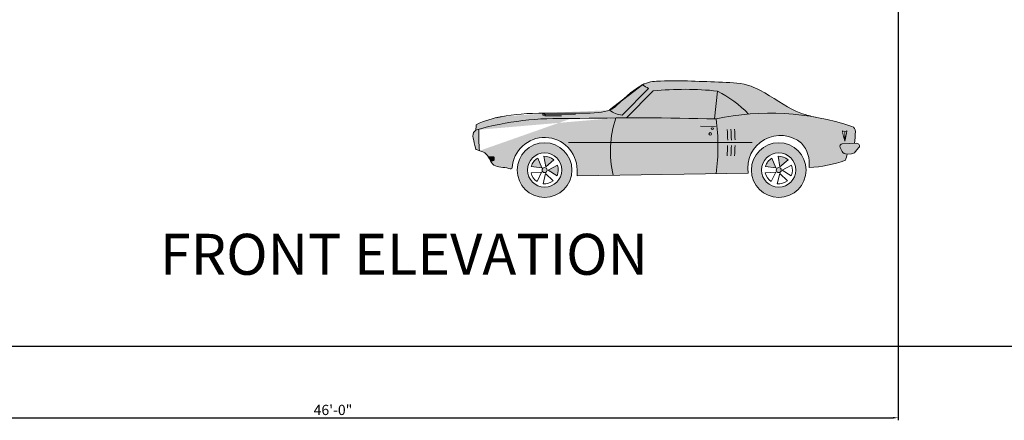
# Model space of a CAD drawing. Units: inches. Extents: x 1662 to 23131, y 1265 to 19127.
# Tile 22 of 26: x 22111 to 22592, y 17831 to 18027. Entities that reach past the tile are written whole.
import ezdxf

# ---------------------------------------------------------------- set-up
doc = ezdxf.new("R2010")
doc.units = ezdxf.units.IN
for name, color, linetype, lineweight in [('A-ANNO-DIMS', 4, 'Continuous', 18), ('A-ANNO-TITL', 7, 'Continuous', 35), ('A-ANNO-TTLB', 7, 'Continuous', 25), ('A-ELEV', 7, 'Continuous', 25), ('A-ELEV-SURF-PATT', 252, 'Continuous', 13), ('A-SITE-VEHC', 8, 'Continuous', 18)]:
    doc.layers.add(name, color=color, linetype=linetype, lineweight=lineweight)
doc.styles.get("Standard").update_dxf_attribs({"font": 'arial.ttf'})
doc.dimstyles.new('ISO-25', dxfattribs={"dimtxt": 5, "dimasz": 2.5, "dimexe": 1.25, "dimexo": 0.625, "dimtad": 1, "dimlunit": 3, "dimtxsty": 'Standard', "dimcen": 2.5, "dimadec": 0, "dimazin": 0, "dimtfac": 1, "dimtmove": 0, "dimatfit": 3, "dimfxl": 1, "dimarcsym": 0})

# ---------------------------------------------------------------- blocks, each defined once
blk = doc.blocks.new('*U125')
for p, q in [((1852.424305694587, 1021.94023515126), (2179.330987173972, 1350.645748622479)), ((1905.028754216457, 986.0402655627327), (2237.281665968954, 1320.121427396675)), ((3032.444313744444, 1318.435483164577), (2995.184084363387, 973.324104566919)), ((1273.239579640142, 1043.030435623248), (871.5032389472328, 1041.001834039635)), ((1098.89508774338, 1012.134004053351), (892.8883415085321, 1010.293803537071)), ((896.6541237575286, 1027.557353910195), (1273.36508552453, 1031.747823418233)), ((2821.704323889107, 882.1853508743229), (3009.40210199737, 879.9097921223942)), ((1184.937477293614, 681.4987119404606), (3461.750511828128, 679.9102527502469)), ((4554.181794982009, 618.5936445548908), (4578.428756696647, 571.2293072468502)), ((4581.292953023774, 664.6633678662108), (4762.788167963406, 670.807787640687)), ((4741.599689284432, 563.0499352002037), (4788.17251968349, 618.8856343936881)), ((189.2120355450149, 502.3517070685087), (247.4549749373119, 502.9995917502729)), ((4638.623553838175, 536.8785697564502), (4696.80346690226, 540.4040575811651)), ((247.9843470866509, 455.4105826600687), (216.7883795485336, 455.0635639533959)), ((263.4603752382749, 487.346356794033), (263.6375820428919, 471.4159829610306)), ((1292.174930811352, 343.511370615137), (1293.022509683079, 267.316507168658))]:
    blk.add_line(p, q)
for points in [[(896.8016502475936, 1014.295153612313), (896.7053017041424, 1022.956606081312, 0.2695324023286518), (892.630915434324, 1029.789683311358), (873.3170212489753, 1040.50624839506, 0.5753831854401361), (867.4395555695834, 1037.001668443855), (867.5359041130301, 1028.340215974855, 0.2695324023286636), (871.6102903828508, 1021.507138744809), (890.9241845682014, 1010.790573661109, 0.5753831854401859)], [(879.7836598367863, 509.3545565197219), (903.1759281139406, 380.3214176471538), (1003.225770169055, 465.0962856635947, 0.1999060696292243)], [(3784.383643640271, 509.3545565197196), (3807.775911917426, 380.3214176471517), (3907.82575397254, 465.0962856635924, 0.1999060696292243)], [(723.7168469426299, 383.4919578957729), (853.6632629200222, 365.8658943225199), (803.9546737544847, 487.2158234763112, 0.1999060696292243)], [(1047.713401858163, 399.8198790703183), (932.2242027500088, 337.699077145239), (1043.766994874665, 268.7428978173945, 0.1999060696292243)], [(3628.316830746115, 383.4919578957707), (3758.263246723507, 365.8658943225165), (3708.554657557972, 487.2158234763079, 0.1999060696292243)], [(3952.313385661648, 399.819879070315), (3836.824186553493, 337.6990771452344), (3948.366978678152, 268.7428978173922, 0.1999060696292243)], [(795.1919940795486, 196.1699165843778), (852.1110275926588, 314.3095490808095), (721.3395879004361, 304.5330618138037, 0.1999060696292243)], [(995.43287725522, 206.2611268358749), (900.664358595724, 296.9014987103449), (869.5517532737088, 169.5093681349639, 0.1999060696292243)], [(3699.791977883036, 196.1699165843755), (3756.711011396144, 314.3095490808073), (3625.939571703921, 304.5330618138014, 0.1999060696292243)], [(3900.032861058707, 206.2611268358726), (3805.264342399209, 296.9014987103415), (3774.151737077194, 169.5093681349606, 0.1999060696292243)]]:
    blk.add_lwpolyline(points, format="xyb", close=True)
for points in [[(4612.178408054545, 697.5855081472733), (4610.911620659674, 811.4659926516836), (4584.21673788074, 823.7136574833391)], [(4612.178408054545, 697.5855081472733), (4610.911620659674, 811.4659926516836), (4637.327449602523, 824.3044521259374)], [(1293.022509683079, 267.316507168658), (3413.278107073423, 300.3593556298297)]]:
    blk.add_lwpolyline(points)
for centre, radius in [((2943.507610451247, 787.54394792536), 15.73283948719639), ((888.3677559944676, 339.0194873812145), 339.0404618073459), ((3792.967739797953, 339.0194873812123), 339.0404618073459), ((888.3677559944676, 339.0194873812145), 212.1199727322649), ((3792.967739797953, 339.0194873812123), 212.1199727322649), ((888.3677559944631, 339.0194873812145), 31.6605939107037), ((3792.967739797948, 339.0194873812123), 31.6605939107037)]:
    blk.add_circle(centre, radius)
for centre, radius, start, end in [((2910.885371335993, 2669.23574072891), 1507.929501774574, 237.6102726860142, 240.9784649091492), ((2627.712114858283, -2413.041321416871), 3753.523683760239, 83.8163327171543, 95.97053738930742), ((2425.838500466955, 99.2748149861123), 1361.735417596019, 43.27478678783127, 63.56652369103386), ((1071.358229971631, -2828.229400839409), 3807.785853883705, 87.83927513879316, 105.8096485545998), ((521.544716666302, -80.01394318122811), 1093.607895506514, 98.53035379505096, 116.1119759439421), ((2034.516407361282, -34648.81188708144), 35635.08741385555, 88.42296055026361, 91.31789804800042), ((1861.480574200575, 1282.39025120185), 260.6074190425228, 230.4240102276009, 268.008535378073), ((3005.128481494482, 571.7965598232081), 1299.348755530903, 161.4307082840575, 193.2363327424058), ((3687.381330221874, -2156.074042366811), 3200.23423309803, 71.52833252843139, 102.1241928632375), ((651.7203661001014, 633.5641918017639), 2387.729331448684, 351.8278966526415, 8.167377222832604), ((4681.26729379385, 819.2266390839337), 63.32118782140739, 357.9320259294628, 71.5283325284308), ((2010.729354338346, 764.8379620713475), 1937.952811191957, 177.5773367925648, 185.5205157003238), ((888.3677559944676, 339.0194873812145), 403.8321575216381, 0.6373223477697438, 176.3412329397426), ((1159.222590401551, 681.5166523895871), 2000.491234107682, 0.8520117729178469, 4.65562176499107), ((1204.825955982183, 682.0239365738142), 2000.491234107682, 0.8520117729178469, 4.65562176499107), ((1250.429321562816, 682.5312207580412), 2000.491234107682, 0.8520117729178469, 4.65562176499107), ((3812.44326471366, 364.6726230309737), 404.3130216030247, 49.22630090364881, 189.1528042882995), ((5492.971123156516, 959.0142065914283), 918.7713379001904, 188.4683166415172, 196.5314518469167), ((3725.788185614365, 939.3563602145823), 918.7713379001904, 344.7431928486226, 352.806328054022), ((2960.464007730524, 881.3625008577552), 1785.245929105045, 353.1942286465509, 357.9320259294632), ((1159.222590401551, 681.5166523895871), 2000.491234107682, 355.2644314046092, 358.8632764442745), ((1204.825955982183, 682.0239365738142), 2000.491234107682, 355.2644314046092, 358.8632764442745), ((1250.429321562816, 682.5312207580412), 2000.491234107682, 355.2644314046092, 358.8632764442745), ((3794.827133462601, 420.2460268887999), 377.0136474469525, 352.7285496129741, 41.66131232724548), ((4582.364191149664, 633.0209018489084), 31.6605939107037, 91.93897627460323, 207.1090160995226), ((4763.859406089295, 639.1653216233844), 31.6605939107037, 320.168349060925, 91.93897627460312), ((247.6310576096746, 487.1702741216726), 15.83029695535184, 0.6373223477697438, 90.63732234776975), ((4634.793549031956, 600.0838218348852), 63.32118782140739, 207.1090160995214, 273.4676724156525), ((2901.892172686372, 940.4796147147171), 1785.245929105045, 344.3985036081313, 346.9384932927042), ((4692.973462096046, 603.6093096596), 63.32118782140739, 273.4676724156508, 320.168349060924), ((247.8082644142905, 471.239900288669), 15.83029695535184, 270.6373223477697, 0.6373223477697438), ((4126.811003434335, 1798.913596362007), 1427.004461663924, 271.6864966331125, 290.2773961774014)]:
    blk.add_arc(centre, radius, start, end)
blk.add_ellipse((2968.963243622841, 853.2791378181013), major_axis=(-16.00108995067517, -0.1779934388400297), ratio=0.6100431599522633)
for points, knots in [([(289.2906990761314, 988.6470416166414), (458.7737514417009, 1020.886061005622), (785.1067050195581, 1067.029451377599), (1645.088223183275, 1018.886905819271), (1784.344214682222, 1140.817014935552), (2091.760888566001, 1431.934919697545), (2519.289461757875, 1455.378874077572), (2948.002349952958, 1431.299395835894), (3379.283347368358, 1419.06290683643), (3689.197264561811, 1266.646942515618), (3901.855848393217, 1112.555284301348), (4093.662622991955, 1033.187703863597), (4189.021814386458, 1009.060173110094), (4249.111677936588, 994.4748246004747)], [18.62982323788346, 18.62982323788346, 18.62982323788346, 18.62982323788346, 19.52740456630144, 20.70057132475832, 21.10798274325262, 21.60856814090276, 21.92335951908455, 23.15135895041792, 23.71617100351322, 23.90874285473794, 24.77794011438314, 24.94307190945345, 25.1877551447545, 25.1877551447545, 25.1877551447545, 25.1877551447545]), ([(485.3586889456344, 364.7896896507493), (482.3269151854019, 360.8630236160399), (469.8642701632046, 350.8862285351804), (389.9323687006885, 380.8945308696264), (233.5219717046482, 354.0424667192036), (184.3560220232451, 564.4315200693248), (76.52041888637723, 575.4467616401544), (33.56437062048743, 599.7488008360459), (16.25711196136743, 683.7323555854283), (-24.37278573086193, 799.8748641589713), (39.13505772293892, 828.9834370117921), (38.00494619388845, 865.2204137053852), (37.84050808420068, 883.8077013151833), (37.78154551397344, 890.4725447213818), (38.61308557628376, 896.5033010551641), (40.21850136081582, 901.9755188649158)], [16.81585287302304, 16.81585287302304, 16.81585287302304, 16.81585287302304, 16.838212158335, 16.88539481137264, 17.18439046154897, 17.47984636192869, 17.65442317330994, 17.67069277424245, 17.69692296666891, 18.01635806820882, 18.05273947455308, 18.14080485493071, 18.14080485493071, 18.14080485493071, 18.17238245689425, 18.17238245689425, 18.17238245689425, 18.17238245689425])]:
    blk.add_open_spline(points, degree=3, knots=knots)
blk = doc.blocks.new('*D257')
at = {"layer": 'A-ANNO-DIMS', "color": 0, "lineweight": -2, "transparency": 16777216}
for p, q in [((21988.149343, 18204.597571), (21988.149343, 17831.289414)), ((22540.149343, 18204.597571), (22540.149343, 17831.289414)), ((21990.649343, 17832.539414), (22537.649343, 17832.539414))]:
    blk.add_line(p, q, dxfattribs=at)
at = {"layer": 'A-ANNO-DIMS', "color": 0, "transparency": 16777216}
for points in [[(21990.649343, 17832.95608066667), (21990.649343, 17832.12274733333), (21988.149343, 17832.539414)], [(22537.649343, 17832.95608066667), (22537.649343, 17832.12274733333), (22540.149343, 17832.539414)]]:
    blk.add_solid(points, dxfattribs=at)
at = {"layer": 'Defpoints', "color": 0, "transparency": 16777216}
for p in [(21988.149343, 18205.222571), (22540.149343, 18205.222571), (22540.149343, 17832.539414)]:
    blk.add_point(p, dxfattribs=at)
at = {"layer": 'A-ANNO-DIMS', "color": 0, "transparency": 16777216, "insert": (22264.149343, 17835.7172789386), "char_height": 5, "attachment_point": 5}
blk.add_mtext('46\'-0"', dxfattribs=at)

msp = doc.modelspace()

# ---------------------------------------------------------------- hatches: boundary and pattern name
at = {"layer": 'A-ELEV-SURF-PATT'}
h = msp.add_hatch(color=256, dxfattribs=at)
h.dxf.hatch_style = 1
h.paths.add_polyline_path([(22452.1564414005, 17966.92818785984), (22399.84911369841, 17966.96468099922, 0.0789795163603548), (22401.02668666265, 17950.94715727827), (22451.21980826151, 17951.72938547417, 0.0405634696086375)])
h.paths.add_polyline_path([(22451.22091017341, 17978.44679475655, 0.0087136791470317), (22402.32747484488, 17978.94051855419, 0.0599818317621977), (22399.84911369841, 17966.96468099922), (22452.1564414005, 17966.92818785984, 0.0307628883025453)], flags=17)
h.paths.add_polyline_path([(22449.01653312292, 17971.15412296394, -1), (22447.77772686408, 17971.15412296394, -1)], flags=16)
edge = h.paths.add_edge_path(flags=16)
edge.add_ellipse((22449.39932027585, 17973.74212256602), major_axis=(0.6299641712865368, 0.0070076157174276), ratio=0.6100431599511486, start_angle=0, end_angle=360)
h.paths.add_polyline_path([(22517.60272427134, 17974.76599696269, 0.1342984033861153), (22451.22091017341, 17978.44679475655, -0.0714154736732145), (22451.21980826151, 17951.72938547417), (22466.89203143532, 17951.97362720428, -0.6997297249664224), (22493.00270443744, 17966.56014157027, -0.2168140947778998), (22496.63733033387, 17954.81488401869, 0.0812964945407138), (22514.45437702691, 17958.27234124313, 0.0110832495234575), (22515.22558053612, 17961.29095805373), (22515.13397815834, 17961.285407288, -0.2979165302681907), (22512.76410425512, 17962.63779852778), (22511.80949946322, 17964.50253621708, -0.5495844291803016), (22512.87686789006, 17966.31630485138), (22518.85471767985, 17966.51868163839, 0.0206754858036655), (22519.30420209342, 17972.31151424214, 0.332637825579096)])
h.paths.add_polyline_path([(22512.99197752894, 17972.57812727778), (22514.04295716706, 17972.09593574844), (22515.08295043253, 17972.60138690885, -0.0351965873901873), (22514.09283068654, 17967.61245210653, -0.0351965873954787)], flags=16)
edge = h.paths.add_edge_path()
edge.add_arc((22412.61007475374, 16576.0220034755), 1402.956197395876, 90.41993816560347, 91.31789804800091)
edge.add_arc((22374.69046147068, 17828.80084151651), 149.9128288930652, 87.83927513879544, 105.176445372924)
edge.add_arc((22411.67357660323, 17970.26018651301), 76.29735477133848, 177.5773367925706, 185.5205157003362)
edge.add_spline(control_points=[(22335.73010304763, 17962.92021584447), (22336.65982734748, 17962.60824091316), (22338.3864516981, 17962.14188753878), (22339.48829724458, 17960.68212267855), (22339.96029633578, 17959.92608198533)], knot_values=[17.37738595315716, 17.37738595315716, 17.37738595315716, 17.37738595315716, 17.49233179028216, 17.59479219905369, 17.59479219905369, 17.59479219905369, 17.59479219905369], degree=3, periodic=0)
edge.add_line((22339.96029633578, 17959.92608198533), (22342.25332544571, 17959.95158925626))
edge.add_arc((22342.26025783438, 17959.32838777482), 0.6232400376125846, 0.637322347675422, 90.63732234767542, ccw=False)
edge.add_line((22342.88345931583, 17959.33532016349), (22342.89043596167, 17958.70814009133))
edge.add_arc((22342.26723448023, 17958.70120770266), 0.6232400376125846, -89.36267765199011, 0.637322347675422, ccw=False)
edge.add_line((22342.27416686891, 17958.07800622122), (22341.04597917056, 17958.06434406741))
edge.add_spline(control_points=[(22341.04597917056, 17958.06434406741), (22341.53983312574, 17957.23082126799), (22343.47249741245, 17954.3906115514), (22347.86267165687, 17955.14430339482), (22351.00959691129, 17953.96287416905), (22351.50025222713, 17954.35566137696), (22351.61961339879, 17954.51025452794)], knot_values=[16.81585287302304, 16.81585287302304, 16.81585287302304, 16.81585287302304, 16.92711796634702, 17.22611361652335, 17.273296269561, 17.29565555487296, 17.29565555487296, 17.29565555487296, 17.29565555487296], degree=3, periodic=0)
edge.add_arc((22367.4861121015, 17953.49567963543), 15.89890383943519, 0.6373223477655756, 176.3412329397391, ccw=False)
edge.add_line((22383.38403236988, 17953.67252543204), (22383.4174016168, 17950.67272765856))
edge.add_line((22383.4174016168, 17950.67272765856), (22401.02668666265, 17950.94715727827))
edge.add_arc((22450.82314853851, 17962.66013130639), 51.15546281617707, 175.1730568004502, 193.2363327424203, ccw=False)
edge.add_arc((22450.82314853851, 17962.66013130638), 51.15546281617626, 161.4426842724245, 175.1730568004336, ccw=False)
edge = h.paths.add_edge_path()
edge.add_arc((22435.96423646621, 17845.14682889536), 147.7765229826732, 83.80965163906188, 95.97053738930572, ccw=False)
edge.add_line((22451.8992577319, 17992.06168805573), (22451.89857500504, 17992.05536450879))
edge.add_arc((22428.01645637208, 17944.0569130057), 53.61163061401374, 43.274786787837, 63.54689059582529, ccw=False)
edge.add_arc((22477.6834969136, 17855.2636509052), 125.9934737440192, 79.89062076904088, 94.84149195846811, ccw=False)
edge.add_spline(control_points=[(22499.79886493387, 17979.30100787241), (22497.43312227442, 17979.87523419169), (22493.67882340061, 17980.82513697726), (22486.12737558177, 17983.94984486851), (22477.75499039156, 17990.0164455856), (22465.55365506897, 17996.01707410217), (22448.5740882416, 17996.49882563759), (22431.69562807644, 17997.44683659198), (22414.86379448621, 17996.52384626206), (22403.49842040932, 17985.76104720403), (22400.80587417094, 17983.35515649412), (22399.26089790273, 17982.72795133468)], knot_values=[20.7750967889878, 20.7750967889878, 20.7750967889878, 20.7750967889878, 21.01978002428886, 21.18491181935917, 22.05410907900436, 22.24668093022908, 22.81149298332438, 24.03949241465776, 24.35428379283954, 24.8548691904897, 25.1877551447545, 25.1877551447545, 25.1877551447545, 25.1877551447545], degree=3, periodic=0)
edge.add_arc((22447.11278987083, 18045.23647701132), 59.36730321945393, 237.6234921527005, 240.978464909164)
edge.add_line((22418.31143618233, 17993.32348521485), (22405.44109437316, 17980.38232324843))
edge.add_arc((22405.79764037734, 17990.63626088822), 10.26013460797703, 230.4240102276183, 268.0085353780588, ccw=False)
edge.add_spline(control_points=[(22399.26089790273, 17982.72795133468), (22398.91501345752, 17982.58753460913), (22392.73024432891, 17980.5167152783), (22365.14308829737, 17982.0610692999), (22352.19454018839, 17980.54941411177), (22346.65770436528, 17979.57742526794)], knot_values=[18.75589005472215, 18.75589005472215, 18.75589005472215, 18.75589005472215, 18.83041551895163, 20.00358227740851, 20.7750967889878, 20.7750967889878, 20.7750967889878, 20.7750967889878], degree=3, periodic=0)
edge.add_arc((22366.81796757324, 17980.97702616026), 0.1558100094039474, 90.18502659585694, 240.6299950219491)
edge.add_arc((22366.97756119335, 17980.63775719173), 0.3116200188072633, 139.2324971502809, 240.9757271361971)
edge.add_line((22366.82636936089, 17980.3652722088), (22367.58675889574, 17979.94336019763))
edge.add_arc((22367.66235481197, 17980.0796026891), 0.1558100094039406, 240.9757271361971, 360.6373223473373)
edge.add_arc((22367.74018303735, 17980.38745761783), 0.3158959182360402, 284.2899236714064, 403.5767128608039)
edge.add_line((22367.96903449512, 17980.60521262106), (22367.8123470528, 17980.60346965626))
edge.add_line((22367.8123470528, 17980.60346965626), (22367.81989207654, 17979.92519407368))
edge.add_line((22367.81989207654, 17979.92519407368), (22367.62267374386, 17979.92343237761))
edge.add_line((22367.62267374386, 17979.92343237761), (22366.66797533241, 17980.4531591931))
edge.add_line((22366.66797533241, 17980.4531591931), (22366.65855420066, 17981.30009140314))
edge.add_spline(control_points=[(22399.26089790273, 17982.72795133468), (22398.91501345752, 17982.58753460913), (22392.73024432891, 17980.5167152783), (22365.14308829737, 17982.0610692999), (22352.19454018839, 17980.54941411177), (22346.65770436528, 17979.57742526794)], knot_values=[18.75589005472215, 18.75589005472215, 18.75589005472215, 18.75589005472215, 18.83041551895163, 20.00358227740851, 20.7750967889878, 20.7750967889878, 20.7750967889878, 20.7750967889878], degree=3, periodic=0)
edge.add_spline(control_points=[(22346.65770436528, 17979.57742526794), (22345.75297573464, 17979.41860059555), (22344.83757370215, 17979.24983629201), (22343.90040119921, 17979.07156759746)], knot_values=[18.62982323788346, 18.62982323788346, 18.62982323788346, 18.62982323788346, 18.75589005472216, 18.75589005472216, 18.75589005472216, 18.75589005472216], degree=3, periodic=0)
edge.add_arc((22353.04426015944, 17936.99830047944), 43.05542895694342, 102.26151830095, 116.1119759438595)
edge.add_spline(control_points=[(22334.09440916317, 17975.65930292219), (22334.03120381732, 17975.44386127614), (22333.99846601959, 17975.20642992442), (22334.00078738062, 17974.94403451473)], knot_values=[18.14080485493071, 18.14080485493071, 18.14080485493071, 18.14080485493071, 18.17238245689425, 18.17238245689425, 18.17238245689425, 18.17238245689425], degree=3, periodic=0)
edge.add_spline(control_points=[(22334.00078738062, 17974.94403451473), (22334.00609279549, 17974.34433610993), (22334.02819553358, 17973.55807482284), (22333.84786860011, 17973.04278712988)], knot_values=[18.06863500429582, 18.06863500429582, 18.06863500429582, 18.06863500429582, 18.14080485493071, 18.14080485493071, 18.14080485493071, 18.14080485493071], degree=3, periodic=0)
edge.add_spline(control_points=[(22335.73010304764, 17962.92021584447), (22335.2477857478, 17963.08206049724), (22334.62810770539, 17963.31046808505), (22333.83243551197, 17963.76061323602), (22333.15104737579, 17967.06705239938), (22331.55144510444, 17971.639592107), (22333.64523379543, 17972.59927200377), (22333.80815129283, 17972.92929415771), (22333.84786860011, 17973.04278712988)], knot_values=[17.59479219905356, 17.59479219905356, 17.59479219905356, 17.59479219905356, 17.65442317330994, 17.67069277424245, 17.69692296666891, 18.01635806820882, 18.05273947455308, 18.06863500429582, 18.06863500429582, 18.06863500429582, 18.06863500429582], degree=3, periodic=0)
edge.add_arc((22374.69046147068, 17828.80084151651), 149.9128288930652, 87.839275138787, 105.80964855459999, ccw=False)
edge.add_arc((22412.61007475372, 16576.02200347548), 1402.956197395896, 90.41993816560228, 91.31789804799871, ccw=False)
edge.add_arc((22412.61007475376, 16576.0220034755), 1402.956197395875, 90.20819683322208, 90.41993816560392, ccw=False)
edge.add_line((22407.51213565355, 17978.96893861896), (22420.59295895089, 17992.12174026596))
h.paths.add_polyline_path([(22380.83416177896, 17953.49567963543, 1), (22354.13806242405, 17953.49567963543, 1)])
h.paths.add_polyline_path([(22359.13493207267, 17953.49567963543, -1), (22375.83729213033, 17953.49567963543, -1)], flags=16)
h.paths.add_polyline_path([(22366.74532459281, 17946.82205289346), (22367.97023031415, 17951.83749110508), (22371.70127435586, 17948.26897252735, -0.1999060696292242)], flags=0)
h.paths.add_polyline_path([(22363.81777501824, 17947.87168078516, -0.1999060696292246), (22360.91019997182, 17952.13794634538), (22366.05868184946, 17952.52284741888)], flags=0)
h.paths.add_polyline_path([(22373.60419237238, 17950.72888477071), (22369.21274386353, 17953.44369498048), (22373.75956272606, 17955.88939584367, -0.1999060696292243)], flags=16)
h.paths.add_polyline_path([(22366.23963202628, 17953.49567963543, -1), (22368.73259217673, 17953.49567963543, -1)], flags=16)
h.paths.add_polyline_path([(22366.11979347652, 17954.5526247906), (22361.00379284749, 17955.24656430136, -0.1999060696292243), (22364.16276240702, 17959.3301810565)], flags=16)
h.paths.add_polyline_path([(22368.06911100384, 17955.12173988212), (22367.14815555986, 17960.20178471963, -0.1999060696292243), (22372.00808116349, 17958.45933311112)], flags=16)
h.paths.add_polyline_path([(22495.18849184996, 17953.49567963543, 1), (22468.49239249505, 17953.49567963543, 1)])
h.paths.add_polyline_path([(22473.48926214367, 17953.49567963543, -1), (22490.19162220133, 17953.49567963543, -1)], flags=16)
h.paths.add_polyline_path([(22481.09965466381, 17946.82205289346), (22482.32456038515, 17951.83749110508), (22486.05560442686, 17948.26897252735, -0.1999060696292243)], flags=0)
h.paths.add_polyline_path([(22478.17210508924, 17947.87168078516, -0.1999060696292246), (22475.26453004282, 17952.13794634538), (22480.41301192047, 17952.52284741888)], flags=0)
h.paths.add_polyline_path([(22480.59396209728, 17953.49567963543, -1), (22483.08692224773, 17953.49567963543, -1)], flags=16)
h.paths.add_polyline_path([(22483.56707393453, 17953.44369498048), (22488.11389279706, 17955.88939584367, -0.1999060696292243), (22487.95852244338, 17950.72888477071)], flags=0)
h.paths.add_polyline_path([(22480.47412354753, 17954.5526247906), (22475.35812291849, 17955.24656430136, -0.1999060696292243), (22478.51709247802, 17959.3301810565)], flags=16)
h.paths.add_polyline_path([(22482.42344107485, 17955.12173988212), (22481.50248563086, 17960.20178471963, -0.1999060696292243), (22486.36241123449, 17958.45933311112)], flags=16)
h = msp.add_hatch(color=256, dxfattribs=at)
h.dxf.hatch_style = 1
edge = h.paths.add_edge_path()
edge.add_arc((22447.11278987083, 18045.23647701132), 59.36730321945393, 237.61027268602828, 240.97846490916402, ccw=False)
edge.add_line((22415.3111856773, 17995.10530245627), (22404.61254705515, 17986.85493282992))
edge.add_spline(control_points=[(22404.61254705518, 17986.85493282995), (22404.34337512708, 17986.6049030321), (22402.01464209999, 17984.43523582182), (22400.80587417094, 17983.35515649412), (22399.26089790273, 17982.72795133467)], knot_values=[20.77509678898748, 20.77509678898748, 20.77509678898748, 20.77509678898748, 20.81638210265321, 21.14926805691834, 21.14926805691834, 21.14926805691834, 21.14926805691834], degree=3, periodic=0)
edge.add_arc((22405.79764037734, 17990.63626088822), 10.26013460797703, 230.4240102276053, 268.0085353780588)
edge.add_line((22405.44109437316, 17980.38232324843), (22418.31143618233, 17993.32348521485))
h = msp.add_hatch(color=256, dxfattribs=at)
h.dxf.hatch_style = 1
h.paths.add_polyline_path([(22451.8992577319, 17992.06168805573, 0.0531117298987124), (22420.59295895089, 17992.12174026596), (22407.51213565355, 17978.96893861896, -0.0076490150394212), (22450.43163684043, 17978.46830235928)])
h.paths.add_polyline_path([(22451.89857500504, 17992.05536450879), (22450.43163684043, 17978.46830235928, -0.0001406968969288), (22451.22091017341, 17978.44679475655, -0.031787477305803), (22467.04971666748, 17980.80758004461, 0.0886851529435796)])
h = msp.add_hatch(color=256, dxfattribs=at)
h.dxf.hatch_style = 1
h.paths.add_polyline_path([(22521.02173271918, 17964.51403188002, 0.6479856101104088), (22520.02234879319, 17966.55821114172), (22512.87686789006, 17966.31630485138, 0.5495844291806617), (22511.80949946322, 17964.50253621707), (22512.76410425512, 17962.63779852778, 0.2979165302682132), (22515.13397815834, 17961.285407288), (22517.42452591677, 17961.42420602126, 0.2066381190142729), (22519.18815671922, 17962.31577600626)])
edge = h.paths.add_edge_path()
edge.add_arc((22374.69046147068, 17828.80084151651), 149.9128288930652, 105.176445372924, 105.8096485545982)
edge.add_spline(control_points=[(22333.84786860011, 17973.04278712988), (22333.80815129283, 17972.92929415771), (22333.64523379543, 17972.59927200377), (22331.55144510444, 17971.639592107), (22333.15104737579, 17967.06705239938), (22333.83243551197, 17963.76061323602), (22334.62810770538, 17963.31046808505), (22335.2477857478, 17963.08206049724), (22335.73010304763, 17962.92021584447)], knot_values=[17.59479219905369, 17.59479219905369, 17.59479219905369, 17.59479219905369, 17.61068772879642, 17.6470691351407, 17.9665042366806, 17.99273442910706, 18.00900403003957, 18.06863500429582, 18.06863500429582, 18.06863500429582, 18.06863500429582], degree=3, periodic=0)
edge.add_arc((22411.67357660323, 17970.26018651301), 76.29735477133848, 177.5773367925706, 185.5205157003333, ccw=False)
h = msp.add_hatch(color=256, dxfattribs=at)
h.dxf.hatch_style = 1
edge = h.paths.add_edge_path()
edge.add_arc((22342.26025783438, 17959.32838777482), 0.6232400376125846, 0.6373223476754206, 90.63732234767544)
edge.add_line((22342.25332544571, 17959.95158925626), (22339.96029633578, 17959.92608198533))
edge.add_spline(control_points=[(22339.96029633578, 17959.92608198533), (22340.33679955468, 17959.32300507282), (22340.68321597821, 17958.67661291418), (22341.04597917056, 17958.06434406741)], knot_values=[17.29565555487296, 17.29565555487296, 17.29565555487296, 17.29565555487296, 17.37738595315716, 17.37738595315716, 17.37738595315716, 17.37738595315716], degree=3, periodic=0)
edge.add_line((22341.04597917056, 17958.06434406741), (22342.27416686891, 17958.07800622122))
edge.add_arc((22342.26723448023, 17958.70120770266), 0.6232400376125844, 270.6373223480099, 360.6373223476754)
edge.add_line((22342.89043596167, 17958.70814009133), (22342.88345931583, 17959.33532016349))

# ---------------------------------------------------------------- linework, layer by layer
at = {"layer": 'A-ANNO-TTLB'}
msp.add_lwpolyline([(21860.9894441816, 19103.60537680307), (23130.85973518679, 19103.60537680307), (23130.85973518679, 17867.35097635912), (21860.9894441816, 17867.35097635912)], close=True, dxfattribs=at)
at = {"layer": 'A-ELEV'}
for q in [(22399.26089790274, 17982.72795133468), (22415.3111856773, 17995.10530245627), (22415.3111856773, 17995.10530245627)]:
    msp.add_line((22415.3111856773, 17995.10530245627), q, dxfattribs=at)

# ---------------------------------------------------------------- block references
at = {"layer": 'A-SITE-VEHC', "xscale": 0.0393700787401575, "yscale": 0.0393700787401575, "zscale": 0.0393700787401575}
msp.add_blockref('*U125', (22332.51100359778, 17940.14845572279), dxfattribs=at)

# ---------------------------------------------------------------- texts
at = {"layer": 'A-ANNO-TITL', "insert": (22179.62525902577, 17922.35456494379), "char_height": 20, "attachment_point": 1}
msp.add_mtext_dynamic_manual_height_columns('FRONT ELEVATION', width=1142.595510895509, gutter_width=12.5, heights=[0], dxfattribs=at)

# ---------------------------------------------------------------- dimensions: what is measured, and where the dimension line sits
at = {"layer": 'A-ANNO-DIMS'}
dim = msp.add_linear_dim(base=(22540.149343, 17832.539414), p1=(21988.149343, 18205.222571), p2=(22540.149343, 18205.222571), dimstyle='ISO-25', override={"dimdec": 1, "dimlfac": 1, "dimrnd": 0, "dimzin": 1, "dimdsep": 46, "dimlunit": 4, "dimfrac": 2}, dxfattribs=at)
dim.commit()
dim.dimension.update_dxf_attribs({"geometry": '*D257', "text_midpoint": (22264.149343, 17835.7172789386)})

doc.saveas('drawing.dxf')
